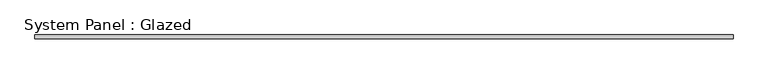
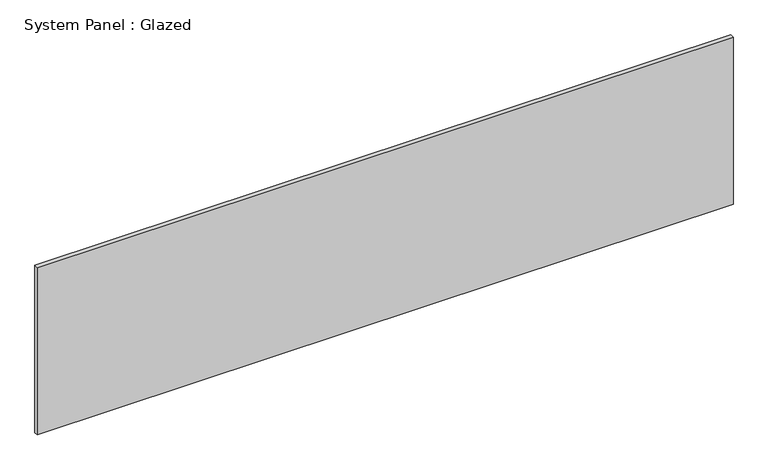
"""IFC4 building model written with IfcOpenShell, lengths in millimetres: plate geometry, System Panel : Glazed."""

from ifc_helpers import new_model, si_unit, origin, origin_with_axes, place, context, project, spatial, polyline, outline, extrude, source, transform, mapped, element, save


def system_panel_glazed_7e85febf(model_context):
    return source(origin(), model_context, "Body", "SweptSolid", [
        extrude(outline(polyline([(2273.9398433, 19.05), (-2273.9398433, 19.05), (-2273.9398433, 44.45), (2273.9398433, 44.45), (2273.9398433, 19.05)])), origin_with_axes(), (0.0, 0.0, 1.0), 1155.7),
    ])


if __name__ == "__main__":
    model = new_model("IFC4")
    model_context = context("Model", 3, world=origin())
    ifc_project = project(units=[si_unit("LENGTHUNIT", "METRE", prefix="MILLI")], contexts=[model_context])
    site = spatial("IfcSite", under=ifc_project)
    building = spatial("IfcBuilding", under=site)
    placement = place(None, origin())
    system_panel_glazed_shape = system_panel_glazed_7e85febf(model_context)
    element("IfcPlate", 1, ObjectType="System Panel : Glazed", at=placement, inside=building, context=model_context, shape_type="MappedRepresentation", body=[
        mapped(system_panel_glazed_shape, transform((0.0, 0.0, 0.0), x_axis=(1.0, 0.0, 0.0), y_axis=(0.0, 1.0, 0.0), z_axis=(0.0, 0.0, 1.0))),
    ])
    save(model, "model.ifc")

# Revit data of these elements
# Type "System Panel : Glazed"
#   Construction Type Id = "GSP4R"
#   Analytic Construction = "1/8 in Pilkington single glazing"
#   Visual Light Transmittance = 0.9
#   Solar Heat Gain Coefficient = 0.86
#   Heat Transfer Coefficient (U) = 1.18115 BTU/(h·ft²·°F)
# Element 1 (IfcPlate, "System Panel : Glazed")
#   Materials on its faces: "Glass"
# Materials
#   "Glass": class "Glass", colour RGB 0 128 192, transparency 0.75, Description = "Soda Lime Glass", Cost = 0
